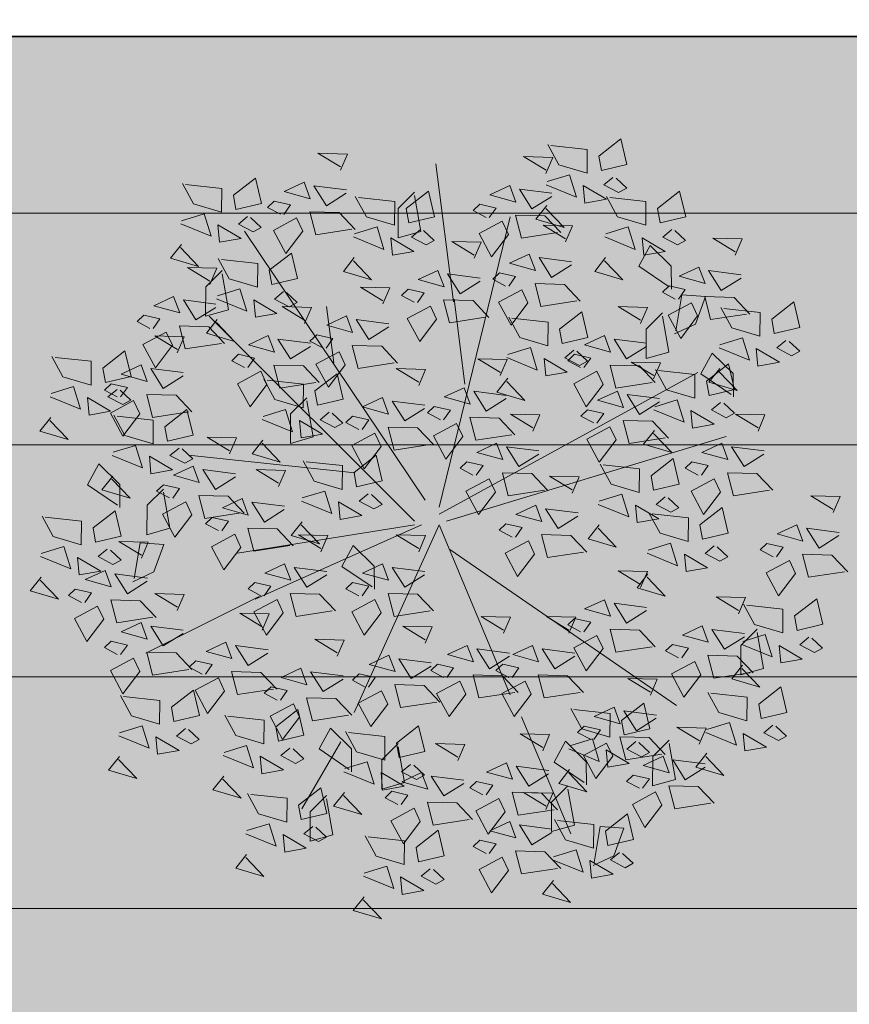
# Model space of a CAD drawing. Units: inches. Extents: x 1704 to 6393, y -157 to 1172.
# Tile 104 of 122: x 2627 to 2654, y 1002 to 1034. Entities that reach past the tile are written whole.
import ezdxf

# ---------------------------------------------------------------- set-up
doc = ezdxf.new("R2010")
doc.units = ezdxf.units.IN
doc.header["$MEASUREMENT"] = 0
for name, color, linetype, lineweight in [('A-ANNO-DIMS', 7, 'Continuous', 13), ('C-PROP', 7, 'Continuous', 35), ('L-DECK-PLNK-PATT', 250, 'Continuous', 13), ('L-shrub', 74, 'Continuous', 18)]:
    doc.layers.add(name, color=color, linetype=linetype, lineweight=lineweight)
doc.layers.add('L-DECK-PATT', color=35, linetype='Continuous', lineweight=13, true_color=0xa6725b)
doc.styles.get("Standard").update_dxf_attribs({"font": 'arial.ttf'})
doc.dimstyles.get("Standard").update_dxf_attribs({"dimtxt": 6, "dimasz": 2, "dimexe": 0.18, "dimexo": 0.0625, "dimgap": 0.09, "dimtad": 0, "dimtih": 1, "dimtoh": 1, "dimdec": 1, "dimzin": 0, "dimdsep": 46, "dimlunit": 3, "dimtxsty": 'Standard', "dimblk": 'ARCHTICK', "dimcen": 0.09, "dimadec": 0, "dimazin": 0, "dimtfac": 1, "dimtdec": 1, "dimtofl": 0, "dimtmove": 0, "dimatfit": 3, "dimfxl": 1, "dimtolj": 1, "dimtzin": 0, "dimarcsym": 0})

# ---------------------------------------------------------------- blocks, each defined once
blk = doc.blocks.new('flower shrub 2')
at = {"layer": 'L-shrub'}
for p, q in [((-106.23, 211.82), (-92.99, 218)), ((-93.69, 216.06), (-97.6, 193.26)), ((-112.6, 194.32), (-106.23, 211.82)), ((71.95, 198.59), (86.43, 202.67)), ((86.43, 202.67), (86.36, 184.05)), ((-97.6, 193.26), (-112.6, 194.32)), ((-81.12, 192.39), (-66.64, 196.47)), ((-66.64, 196.47), (-66.71, 177.85)), ((75.99, 175.82), (71.95, 198.59)), ((-77.07, 169.62), (-81.12, 192.39)), ((86.36, 184.05), (75.99, 173.75)), ((-66.71, 177.85), (-77.08, 167.55)), ((26.45, 165.53), (40.92, 169.61)), ((40.92, 169.61), (40.85, 150.99)), ((-145.24, 163.47), (-130.76, 167.54)), ((-141.2, 140.7), (-145.24, 163.47)), ((-130.76, 167.54), (-130.83, 148.93)), ((-88.72, 152.29), (-88.87, 166.9)), ((-87.4, 165.46), (-68.26, 152.47)), ((30.49, 142.76), (26.45, 165.53)), ((60.21, 144.02), (60.06, 158.64)), ((61.53, 157.19), (80.67, 144.21)), ((-75.44, 139.25), (-88.72, 152.29)), ((-68.26, 152.47), (-75.44, 139.25)), ((40.85, 150.99), (30.48, 140.69)), ((-130.83, 148.93), (-141.21, 138.63)), ((73.5, 130.99), (60.21, 144.02)), ((80.67, 144.21), (73.5, 130.99)), ((-201.09, 93.22), (-186.61, 97.3)), ((-186.61, 97.3), (-186.68, 78.69)), ((-197.05, 70.45), (-201.09, 93.22)), ((-186.68, 78.69), (-197.06, 68.38)), ((45.73, 28.33), (45.58, 42.95)), ((47.06, 41.5), (66.19, 28.51)), ((185.43, 32.08), (198.67, 38.26)), ((179.06, 14.59), (185.43, 32.08)), ((197.96, 36.32), (194.06, 13.53)), ((59.02, 15.29), (45.73, 28.33)), ((66.19, 28.51), (59.02, 15.29)), ((194.06, 13.53), (179.06, 14.59)), ((175.38, 4.39), (189.86, 8.47)), ((189.86, 8.47), (189.78, -10.15)), ((179.42, -18.38), (175.38, 4.39)), ((189.78, -10.15), (179.41, -20.45)), ((207.07, -23.32), (206.92, -8.7)), ((208.4, -10.15), (227.53, -23.13)), ((220.36, -36.35), (207.07, -23.32)), ((227.53, -23.13), (220.36, -36.35)), ((84.36, -53.46), (98.84, -49.38)), ((98.84, -49.38), (98.77, -68)), ((88.41, -76.23), (84.36, -53.46)), ((98.77, -68), (88.4, -78.3)), ((-181.81, -93.56), (-181.96, -78.94)), ((-180.48, -80.39), (-161.34, -93.38)), ((-168.52, -106.6), (-181.81, -93.56)), ((-161.34, -93.38), (-168.52, -106.6)), ((-141.1, -107.17), (-126.62, -103.09)), ((-126.62, -103.09), (-126.7, -121.71)), ((-137.06, -129.94), (-141.1, -107.17)), ((-157.94, -124.93), (-144.7, -118.75)), ((-145.41, -120.69), (-149.31, -143.48)), ((-126.7, -121.71), (-137.07, -132.01)), ((-164.31, -142.42), (-157.94, -124.93)), ((138.15, -134.03), (152.62, -129.95)), ((152.62, -129.95), (152.55, -148.57)), ((142.19, -156.8), (138.15, -134.03)), ((-149.31, -143.48), (-164.31, -142.42)), ((-142.51, -161.74), (-142.65, -147.12)), ((-141.18, -148.57), (-122.04, -161.55)), ((152.55, -148.57), (142.18, -158.87)), ((-129.22, -174.77), (-142.51, -161.74)), ((-122.04, -161.55), (-129.22, -174.77)), ((16.1, -183.61), (30.58, -179.53)), ((30.58, -179.53), (30.51, -198.15)), ((20.14, -206.38), (16.1, -183.61)), ((30.51, -198.15), (20.14, -208.45))]:
    blk.add_line(p, q, dxfattribs=at)
for points in [[(52.15, 237.83), (59.05, 246.56), (41.2, 251.84), (52.74, 239.81)], [(-67.82, 227.5), (-60.92, 236.23), (-78.77, 241.51), (-67.23, 229.48)], [(-39.32, 221.12), (-28.59, 235.29), (-20.71, 220.61), (-35.41, 212.74), (-39.32, 221.12)], [(29.03, 225.28), (27.99, 236.36), (14.33, 233.94), (29.03, 225.28)], [(52.02, 222.79), (37.77, 218.39), (33.35, 232.62), (52.6, 224.77)], [(-90.95, 214.95), (-91.98, 226.03), (-105.64, 223.61), (-90.95, 214.95)], [(10.23, 220.07), (15.95, 224.84), (6.62, 229.76), (1.48, 226.97), (8.24, 220.66)], [(126.62, 210.97), (133.52, 219.7), (115.67, 224.99), (127.2, 212.95)], [(-109.75, 209.74), (-104.02, 214.51), (-113.35, 219.43), (-118.49, 216.64), (-111.73, 210.33)], [(-67.96, 212.46), (-82.2, 208.06), (-86.62, 222.29), (-67.37, 214.44)], [(-70.39, 219.89), (-47.54, 223.41), (-43.79, 208.84), (-62.4, 209.34), (-72.46, 219.95)], [(19.2, 206.65), (5.18, 195.71), (1.34, 211.93), (17.57, 215.74), (19.2, 206.65)], [(49.53, 199.82), (26.54, 202.32), (26.68, 217.36), (44.53, 212.08), (51.52, 199.24)], [(-70.44, 189.49), (-93.43, 191.99), (-93.29, 207.03), (-75.44, 201.75), (-68.45, 188.91)], [(-27.19, 210.46), (-31.5, 204.37), (-21.21, 202.03), (-16.97, 206.05), (-25.13, 210.4)], [(103.49, 198.43), (102.46, 209.5), (88.8, 207.08), (103.49, 198.43)], [(-100.78, 196.32), (-114.8, 185.38), (-118.63, 201.6), (-102.4, 205.41), (-100.78, 196.32)], [(-66.87, 197.06), (-54.24, 204.99), (-46.3, 192.37), (-66.93, 195)], [(-44.01, 200.58), (-40.16, 190.14), (-27.58, 196), (-44.01, 200.58)], [(16.53, 190.13), (27.26, 204.31), (35.14, 189.63), (20.44, 181.76), (16.53, 190.13)], [(84.69, 193.22), (90.42, 197.99), (81.09, 202.9), (75.95, 200.11), (82.71, 193.8)], [(126.48, 195.93), (112.24, 191.53), (107.82, 205.76), (127.07, 197.91)], [(-136.54, 179.8), (-125.81, 193.98), (-117.93, 179.3), (-132.63, 171.43), (-136.54, 179.8)], [(-47.57, 123.92), (-79, 197.93)], [(-37.25, 183.93), (-26.52, 198.11), (-18.64, 183.43), (-33.34, 175.56), (-37.25, 183.93)], [(-14.54, 188.9), (8.31, 192.42), (12.06, 177.85), (-6.55, 178.35), (-16.61, 188.96)], [(93.66, 179.79), (79.64, 168.86), (75.81, 185.07), (92.04, 188.89), (93.66, 179.79)], [(124, 172.97), (101.01, 175.46), (101.15, 190.5), (119, 185.22), (125.98, 172.38)], [(-167.61, 178.57), (-144.76, 182.09), (-141.01, 167.52), (-159.62, 168.02), (-169.68, 178.63)], [(-68.32, 182.7), (-45.47, 186.22), (-41.72, 171.65), (-60.33, 172.15), (-70.39, 182.76)], [(-63.13, 182.49), (-67.54, 172.28), (-48.93, 171.78), (-63.18, 180.43)], [(64.56, 171.72), (71.46, 180.45), (53.61, 185.73), (65.15, 173.7)], [(66.94, 139.62), (91.63, 182.23)], [(28.66, 179.47), (24.35, 173.38), (34.64, 171.04), (38.88, 175.06), (30.72, 179.41)], [(141.1, 161.39), (148, 170.12), (130.14, 175.4), (141.68, 163.37)], [(-124.41, 169.14), (-128.72, 163.05), (-118.43, 160.71), (-114.19, 164.73), (-122.34, 169.08)], [(-78.16, 157.26), (-71.26, 165.99), (-89.12, 171.27), (-77.58, 159.24)], [(-25.12, 173.27), (-29.43, 167.19), (-19.14, 164.84), (-14.9, 168.86), (-23.06, 173.21)], [(-11.02, 166.07), (1.61, 174), (9.54, 161.38), (-11.08, 164.01)], [(11.84, 169.59), (15.69, 159.15), (28.27, 165.01), (11.84, 169.59)], [(41.44, 159.17), (40.4, 170.25), (26.74, 167.83), (41.44, 159.17)], [(-164.09, 155.74), (-151.46, 163.67), (-143.52, 151.05), (-164.15, 153.68)], [(-105.51, 148.81), (-94.78, 162.99), (-86.9, 148.31), (-101.6, 140.44), (-105.51, 148.81)], [(-64.8, 159.87), (-52.17, 167.8), (-44.24, 155.19), (-64.86, 157.81)], [(-41.95, 163.39), (-38.09, 152.95), (-25.52, 158.81), (-41.95, 163.39)], [(22.64, 153.96), (28.36, 158.73), (19.03, 163.65), (13.89, 160.86), (20.65, 154.55)], [(64.43, 156.68), (50.18, 152.28), (45.76, 166.51), (65.01, 158.66)], [(207.29, 148.99), (214.19, 157.72), (196.34, 163.01), (207.88, 150.97)], [(-165.04, 146.93), (-158.14, 155.66), (-175.99, 160.94), (-164.45, 148.91)], [(-141.23, 159.26), (-137.38, 148.82), (-124.8, 154.68), (-141.23, 159.26)], [(117.97, 148.84), (116.93, 159.92), (103.28, 157.5), (117.97, 148.84)], [(140.96, 146.35), (126.72, 141.95), (122.3, 156.18), (141.55, 148.33)], [(-136.58, 147.58), (-113.73, 151.1), (-109.98, 136.53), (-128.59, 137.03), (-138.65, 147.64)], [(-101.29, 144.71), (-102.33, 155.79), (-115.98, 153.37), (-101.29, 144.71)], [(-78.3, 142.22), (-92.54, 137.81), (-96.96, 152.05), (-77.71, 144.2)], [(-7.28, 151.5), (-11.69, 141.29), (6.92, 140.79), (-7.33, 149.44)], [(61.95, 133.71), (38.95, 136.21), (39.09, 151.25), (56.94, 145.97), (63.93, 133.13)], [(99.17, 143.63), (104.9, 148.4), (95.57, 153.32), (90.43, 150.53), (97.19, 144.22)], [(-188.17, 134.38), (-189.2, 145.46), (-202.86, 143.04), (-188.17, 134.38)], [(-120.09, 139.5), (-114.36, 144.27), (-123.69, 149.19), (-128.83, 146.4), (-122.07, 140.09)], [(-61.06, 145.31), (-65.47, 135.09), (-46.86, 134.59), (-61.11, 143.24)], [(31.61, 140.54), (17.59, 129.6), (13.76, 145.82), (29.99, 149.63), (31.61, 140.54)], [(184.16, 136.45), (183.13, 147.53), (169.47, 145.1), (184.16, 136.45)], [(207.15, 133.95), (192.91, 129.55), (188.49, 143.78), (207.74, 135.93)], [(-206.97, 129.17), (-201.24, 133.94), (-210.57, 138.86), (-215.71, 136.07), (-208.95, 129.76)], [(-165.18, 131.89), (-179.42, 127.48), (-183.84, 141.72), (-164.59, 133.87)], [(-160.34, 141.17), (-164.76, 130.96), (-146.15, 130.46), (-160.4, 139.11)], [(-93.39, 138.15), (-97.69, 132.06), (-87.4, 129.72), (-83.16, 133.74), (-91.32, 138.09)], [(108.14, 130.21), (94.12, 119.27), (90.29, 135.49), (106.52, 139.3), (108.14, 130.21)], [(93.06, 124.02), (103.79, 138.2), (111.67, 123.52), (96.98, 115.65), (93.06, 124.02)], [(138.48, 123.38), (115.49, 125.88), (115.63, 140.92), (133.48, 135.64), (140.46, 122.8)], [(165.36, 131.24), (171.09, 136.01), (161.76, 140.92), (156.62, 138.13), (163.38, 131.82)], [(-133.06, 124.75), (-120.43, 132.68), (-112.5, 120.06), (-133.12, 122.69)], [(-111.12, 126.07), (-125.14, 115.14), (-128.97, 131.36), (-112.74, 135.17), (-111.12, 126.07)], [(-80.78, 119.25), (-103.77, 121.75), (-103.63, 136.79), (-85.78, 131.5), (-78.8, 118.66)], [(-198, 115.75), (-212.02, 104.81), (-215.85, 121.03), (-199.62, 124.84), (-198, 115.75)], [(-167.66, 108.92), (-190.65, 111.42), (-190.51, 126.46), (-172.66, 121.17), (-165.67, 108.33)], [(-110.21, 128.27), (-106.35, 117.83), (-93.78, 123.69), (-110.21, 128.27)], [(37.21, 115.75), (47.94, 129.93), (55.82, 115.25), (41.13, 107.38), (37.21, 115.75)], [(61.99, 122.79), (84.85, 126.31), (88.59, 111.74), (69.98, 112.24), (59.92, 122.85)], [(174.33, 117.81), (160.31, 106.88), (156.48, 123.09), (172.71, 126.91), (174.33, 117.81)], [(204.67, 110.99), (181.68, 113.48), (181.82, 128.52), (199.67, 123.24), (206.65, 110.4)], [(-53.8, 109.56), (-43.07, 123.73), (-35.19, 109.05), (-49.89, 101.18), (-53.8, 109.56)], [(-12.43, 109.56), (-1.7, 123.73), (6.18, 109.05), (-8.52, 101.18), (-12.43, 109.56)], [(4.49, 2.24), (58.38, 121.09)], [(140.64, 107.49), (151.37, 121.67), (159.25, 106.99), (144.55, 99.12), (140.64, 107.49)], [(-2.25, 17.94), (-145.94, 116.61)], [(6.14, 114.53), (29, 118.04), (32.74, 103.47), (14.13, 103.98), (4.07, 114.58)], [(105.19, 113.36), (100.89, 107.27), (111.17, 104.93), (115.42, 108.95), (107.26, 113.3)], [(-161.36, 97.16), (-150.63, 111.34), (-142.75, 96.66), (-157.45, 88.79), (-161.36, 97.16)], [(-129.32, 110.18), (-133.73, 99.97), (-115.12, 99.47), (-129.37, 108.12)], [(-84.87, 108.33), (-62.02, 111.85), (-58.27, 97.28), (-76.88, 97.78), (-86.94, 108.38)], [(-43.5, 108.33), (-20.65, 111.85), (-16.9, 97.28), (-35.51, 97.78), (-45.57, 108.38)], [(4.49, 2.24), (-40.41, 109.88)], [(65.51, 99.96), (78.14, 107.89), (86.08, 95.27), (65.46, 97.9)], [(109.57, 106.26), (132.42, 109.78), (136.17, 95.21), (117.56, 95.71), (107.5, 106.32)], [(194.42, 95.09), (205.15, 109.27), (213.03, 94.59), (198.33, 86.72), (194.42, 95.09)], [(-187.79, 91.15), (-180.89, 99.88), (-198.75, 105.16), (-187.21, 93.13)], [(49.34, 105.09), (45.04, 99.01), (55.32, 96.67), (59.57, 100.68), (51.41, 105.04)], [(88.37, 103.48), (92.23, 93.04), (104.8, 98.9), (88.37, 103.48)], [(-192.43, 95.93), (-169.58, 99.45), (-165.83, 84.88), (-184.44, 85.38), (-194.5, 95.99)], [(-99.31, 80.63), (-88.58, 94.81), (-80.7, 80.13), (-95.39, 72.26), (-99.31, 80.63)], [(-41.67, 98.9), (-45.98, 92.81), (-35.69, 90.47), (-31.45, 94.49), (-39.6, 98.84)], [(-0.3, 98.9), (-4.61, 92.81), (5.68, 90.47), (9.92, 94.49), (1.76, 98.84)], [(9.66, 91.7), (22.29, 99.62), (30.23, 87.01), (9.61, 89.63)], [(32.52, 95.21), (36.38, 84.78), (48.95, 90.64), (32.52, 95.21)], [(152.77, 96.83), (148.46, 90.75), (158.75, 88.4), (162.99, 92.42), (154.83, 96.77)], [(163.35, 93.87), (186.2, 97.38), (189.95, 82.82), (171.34, 83.32), (161.28, 93.92)], [(-210.92, 78.6), (-211.96, 89.68), (-225.62, 87.26), (-210.92, 78.6)], [(-81.35, 85.5), (-68.72, 93.43), (-60.78, 80.81), (-81.41, 83.43)], [(-58.49, 89.02), (-54.64, 78.58), (-42.06, 84.44), (-58.49, 89.02)], [(-39.98, 85.5), (-27.35, 93.43), (-19.41, 80.81), (-40.04, 83.43)], [(-17.12, 89.02), (-13.27, 78.58), (-0.69, 84.44), (-17.12, 89.02)], [(113.09, 83.43), (125.72, 91.36), (133.65, 78.75), (113.03, 81.37)], [(-229.72, 73.39), (-223.99, 78.16), (-233.32, 83.08), (-238.46, 80.29), (-231.7, 73.98)], [(-187.93, 76.11), (-202.17, 71.7), (-206.59, 85.94), (-187.34, 78.09)], [(-149.23, 86.5), (-153.54, 80.42), (-143.25, 78.07), (-139.01, 82.09), (-147.17, 86.44)], [(-130.38, 79.41), (-107.52, 82.92), (-103.78, 68.35), (-122.39, 68.86), (-132.45, 79.46)], [(69.26, 85.39), (64.84, 75.18), (83.45, 74.68), (69.2, 83.33)], [(118.58, 47.68), (190.43, 83.56)], [(135.94, 86.95), (139.8, 76.51), (152.38, 82.37), (135.94, 86.95)], [(206.55, 84.43), (202.24, 78.35), (212.53, 76.01), (216.77, 80.02), (208.61, 84.38)], [(-188.91, 73.1), (-176.28, 81.03), (-168.35, 68.42), (-188.97, 71.04)], [(-166.05, 76.62), (-162.2, 66.18), (-149.62, 72.04), (-166.05, 76.62)], [(13.41, 77.13), (8.99, 66.92), (27.6, 66.41), (13.35, 75.06)], [(166.87, 71.04), (179.5, 78.96), (187.44, 66.35), (166.81, 68.97)], [(217.17, 62.04), (227.9, 76.22), (235.78, 61.54), (221.08, 53.67), (217.17, 62.04)], [(-220.75, 59.96), (-234.77, 49.03), (-238.6, 65.25), (-222.37, 69.06), (-220.75, 59.96)], [(-190.41, 53.14), (-213.4, 55.64), (-213.26, 70.68), (-195.41, 65.39), (-188.43, 52.55)], [(-87.18, 69.97), (-91.48, 63.89), (-81.2, 61.54), (-76.95, 65.56), (-85.11, 69.92)], [(-77.6, 70.93), (-82.02, 60.72), (-63.41, 60.22), (-77.66, 68.87)], [(-36.23, 70.93), (-40.65, 60.72), (-22.04, 60.22), (-36.29, 68.87)], [(41.35, 57.91), (52.08, 72.09), (59.96, 57.41), (45.26, 49.54), (41.35, 57.91)], [(103.41, 57.91), (114.13, 72.09), (122.01, 57.41), (107.32, 49.54), (103.41, 57.91)], [(116.83, 68.87), (112.42, 58.65), (131.03, 58.15), (116.78, 66.8)], [(189.73, 74.55), (193.58, 64.12), (206.16, 69.98), (189.73, 74.55)], [(-126.86, 56.58), (-114.23, 64.5), (-106.29, 51.89), (-126.91, 54.51)], [(186.1, 60.81), (208.96, 64.33), (212.7, 49.76), (194.09, 50.26), (184.03, 60.87)], [(-185.17, 58.54), (-189.58, 48.32), (-170.97, 47.82), (-185.22, 56.47)], [(-104, 60.09), (-100.14, 49.66), (-87.57, 55.52), (-104, 60.09)], [(10.28, 56.68), (33.14, 60.2), (36.88, 45.63), (18.27, 46.13), (8.21, 56.74)], [(72.33, 56.68), (95.19, 60.2), (98.94, 45.63), (80.33, 46.13), (70.27, 56.74)], [(170.61, 56.47), (166.2, 46.26), (184.81, 45.75), (170.56, 54.41)], [(229.3, 51.38), (225, 45.3), (235.28, 42.95), (239.53, 46.97), (231.37, 51.32)], [(-221.35, 33.12), (-210.62, 47.29), (-202.74, 32.61), (-217.44, 24.74), (-221.35, 33.12)], [(-127.81, 33.3), (-120.91, 42.03), (-138.76, 47.31), (-127.22, 35.28)], [(15.72, 2.24), (121.24, 49.33)], [(53.48, 47.25), (49.18, 41.16), (59.46, 38.82), (63.71, 42.84), (55.55, 47.19)], [(115.53, 47.25), (111.23, 41.16), (121.51, 38.82), (125.76, 42.84), (117.6, 47.19)], [(189.62, 37.98), (202.25, 45.91), (210.19, 33.29), (189.57, 35.92)], [(256.93, 35.37), (263.83, 44.1), (245.98, 49.38), (257.52, 37.35)], [(-123.11, 42.01), (-127.53, 31.79), (-108.92, 31.29), (-123.17, 39.94)], [(13.8, 33.85), (26.43, 41.78), (34.37, 29.16), (13.74, 31.79)], [(75.86, 33.85), (88.48, 41.78), (96.42, 29.16), (75.8, 31.79)], [(212.48, 41.5), (216.34, 31.06), (228.91, 36.92), (212.48, 41.5)], [(-252.42, 31.89), (-229.56, 35.41), (-225.82, 20.84), (-244.43, 21.34), (-254.49, 31.94)], [(-150.93, 20.75), (-151.97, 31.83), (-165.63, 29.41), (-150.93, 20.75)], [(-55.87, 20.72), (-45.14, 34.9), (-37.26, 20.22), (-51.96, 12.35), (-55.87, 20.72)], [(36.66, 37.37), (40.51, 26.93), (53.09, 32.79), (36.66, 37.37)], [(98.71, 37.37), (102.57, 26.93), (115.14, 32.79), (98.71, 37.37)], [(233.81, 22.82), (232.77, 33.9), (219.11, 31.48), (233.81, 22.82)], [(-169.73, 15.55), (-164.01, 20.31), (-173.34, 25.23), (-178.48, 22.44), (-171.72, 16.13)], [(-127.94, 18.26), (-142.19, 13.86), (-146.61, 28.09), (-127.36, 20.24)], [(130.3, 16.59), (141.02, 30.77), (148.91, 16.09), (134.21, 8.22), (130.3, 16.59)], [(215.01, 17.61), (220.73, 22.38), (211.4, 27.3), (206.26, 24.51), (213.02, 18.2)], [(256.8, 20.33), (242.55, 15.92), (238.13, 30.16), (257.38, 22.31)], [(-209.22, 22.46), (-213.52, 16.37), (-203.24, 14.03), (-198.99, 18.05), (-207.15, 22.4)], [(-86.94, 19.49), (-64.08, 23.01), (-60.34, 8.44), (-78.95, 8.94), (-89.01, 19.55)], [(17.55, 19.28), (13.13, 9.07), (31.74, 8.57), (17.49, 17.22)], [(20.21, 2.24), (132.47, 20.18)], [(79.6, 19.28), (75.19, 9.07), (93.8, 8.57), (79.54, 17.22)], [(99.22, 15.36), (122.08, 18.88), (125.83, 4.31), (107.22, 4.81), (97.16, 15.42)], [(193.37, 23.42), (188.95, 13.2), (207.56, 12.7), (193.31, 21.35)], [(-248.9, 9.06), (-236.27, 16.99), (-228.33, 4.37), (-248.95, 7)], [(-226.04, 12.58), (-222.18, 2.14), (-209.61, 8), (-226.04, 12.58)], [(-130.42, -4.7), (-153.42, -2.21), (-153.28, 12.83), (-135.43, 7.55), (-128.44, -5.29)], [(-96.78, 2.31), (-89.88, 11.04), (-107.73, 16.33), (-96.19, 4.29)], [(91.45, 0.25), (98.35, 8.98), (80.5, 14.26), (92.04, 2.23)], [(223.98, 4.18), (209.96, -6.75), (206.13, 9.47), (222.35, 13.28), (223.98, 4.18)], [(254.32, -2.64), (231.32, -0.14), (231.46, 14.9), (249.31, 9.61), (256.3, -3.23)], [(-160.76, 2.12), (-174.78, -8.81), (-178.61, 7.4), (-162.38, 11.22), (-160.76, 2.12)], [(-43.74, 10.06), (-48.04, 3.98), (-37.76, 1.63), (-33.51, 5.65), (-41.67, 10)], [(161.32, -4.07), (172.05, 10.11), (179.93, -4.57), (165.24, -12.44), (161.32, -4.07)], [(0, 0), (-177.37, -53.82)], [(-119.91, -10.23), (-120.94, 0.84), (-134.6, -1.58), (-119.91, -10.23)], [(-83.42, -3.34), (-70.79, 4.59), (-62.85, -8.02), (-83.47, -5.4)], [(-60.56, 0.18), (-56.71, -10.26), (-44.13, -4.4), (-60.56, 0.18)], [(20.21, 0), (150.43, -130.06)], [(102.75, -7.47), (115.38, 0.46), (123.31, -12.16), (102.69, -9.53)], [(142.42, 5.93), (138.12, -0.16), (148.4, -2.5), (152.65, 1.52), (144.49, 5.87)], [(-245.15, -5.51), (-249.57, -15.72), (-230.96, -16.22), (-245.21, -7.57)], [(-173.77, -18.53), (-163.04, -4.35), (-155.16, -19.03), (-169.86, -26.9), (-173.77, -18.53)], [(4.49, -4.48), (-159.41, -94.18)], [(-138.71, -15.44), (-132.98, -10.67), (-142.31, -5.76), (-147.45, -8.55), (-140.69, -14.86)], [(-96.92, -12.73), (-111.16, -17.13), (-115.58, -2.9), (-96.33, -10.75)], [(-31.05, -18.53), (-20.32, -4.35), (-12.44, -19.03), (-27.13, -26.9), (-31.05, -18.53)], [(68.33, -12.3), (67.29, -1.22), (53.63, -3.64), (68.33, -12.3)], [(91.32, -14.79), (77.07, -19.2), (72.66, -4.96), (91.9, -12.81)], [(125.6, -3.95), (129.46, -14.39), (142.03, -8.53), (125.6, -3.95)], [(130.25, -5.3), (153.11, -1.78), (156.85, -16.35), (138.24, -15.85), (128.18, -5.24)], [(4.49, -8.97), (-40.41, -192.85)], [(49.53, -17.51), (55.25, -12.74), (45.92, -7.82), (40.78, -10.61), (47.54, -16.92)], [(-204.84, -19.76), (-181.99, -16.24), (-178.24, -30.81), (-196.85, -30.31), (-206.91, -19.7)], [(-99.4, -35.69), (-122.39, -33.2), (-122.25, -18.16), (-104.4, -23.44), (-97.41, -36.28)], [(-79.67, -17.9), (-84.09, -28.12), (-65.48, -28.62), (-79.73, -19.97)], [(-62.12, -19.76), (-39.26, -16.24), (-35.52, -30.81), (-54.13, -30.31), (-64.19, -19.7)], [(13.47, -13.45), (127.98, -183.88)], [(173.45, -14.73), (169.15, -20.81), (179.43, -23.16), (183.68, -19.14), (175.52, -14.79)], [(211.43, -28.68), (218.32, -19.95), (200.47, -14.66), (212.01, -26.7)], [(-129.74, -28.87), (-143.76, -39.8), (-147.59, -23.59), (-131.36, -19.77), (-129.74, -28.87)], [(58.5, -30.94), (44.48, -41.87), (40.65, -25.65), (56.88, -21.84), (58.5, -30.94)], [(88.84, -37.76), (65.84, -35.27), (65.98, -20.22), (83.83, -25.51), (90.82, -38.35)], [(106.49, -22.04), (102.08, -32.25), (120.69, -32.75), (106.44, -24.1)], [(133.77, -28.13), (146.4, -20.2), (154.34, -32.82), (133.72, -30.19)], [(156.63, -24.61), (160.49, -35.05), (173.06, -29.19), (156.63, -24.61)], [(-161.65, -29.19), (-165.95, -35.28), (-155.67, -37.62), (-151.42, -33.6), (-159.58, -29.25)], [(-18.92, -29.19), (-23.22, -35.28), (-12.94, -37.62), (-8.69, -33.6), (-16.85, -29.25)], [(57.96, -30.81), (163.48, -42.02)], [(188.3, -41.22), (187.26, -30.14), (173.6, -32.57), (188.3, -41.22)], [(-201.32, -42.59), (-188.69, -34.66), (-180.76, -47.28), (-201.38, -44.65)], [(-107.58, -51.59), (-96.85, -37.41), (-88.97, -52.09), (-103.67, -59.96), (-107.58, -51.59)], [(-58.6, -42.59), (-45.97, -34.66), (-38.03, -47.28), (-58.65, -44.65)], [(41.35, -47.45), (52.08, -33.28), (59.96, -47.96), (45.26, -55.83), (41.35, -47.45)], [(116.28, -51.4), (123.17, -42.67), (105.32, -37.39), (116.86, -49.42)], [(169.5, -46.43), (175.23, -41.66), (165.89, -36.75), (160.76, -39.54), (167.52, -45.85)], [(211.29, -43.72), (197.04, -48.12), (192.63, -33.89), (211.88, -41.74)], [(-178.47, -39.07), (-174.61, -49.51), (-162.04, -43.65), (-178.47, -39.07)], [(-131.94, -57.6), (-125.04, -48.87), (-142.9, -43.59), (-131.36, -55.62)], [(-35.74, -39.07), (-31.88, -49.51), (-19.31, -43.65), (-35.74, -39.07)], [(-10.36, -53.65), (0.37, -39.48), (8.25, -54.15), (-6.45, -62.02), (-10.36, -53.65)], [(137.52, -42.69), (133.1, -52.91), (151.71, -53.41), (137.46, -44.76)], [(-138.65, -52.81), (-115.8, -49.3), (-112.05, -63.87), (-130.66, -63.36), (-140.72, -52.76)], [(10.28, -48.68), (33.14, -45.17), (36.88, -59.73), (18.27, -59.23), (8.21, -48.63)], [(208.81, -66.68), (185.82, -64.19), (185.95, -49.15), (203.81, -54.43), (210.79, -67.27)], [(-41.43, -54.88), (-18.58, -51.36), (-14.83, -65.93), (-33.44, -65.43), (-43.5, -54.82)], [(93.15, -63.95), (92.11, -52.87), (78.45, -55.29), (93.15, -63.95)], [(178.47, -59.86), (164.45, -70.79), (160.62, -54.58), (176.85, -50.76), (178.47, -59.86)], [(194.42, -68.11), (205.15, -53.94), (213.03, -68.62), (198.33, -76.49), (194.42, -68.11)], [(250.73, -65.86), (257.63, -57.13), (239.78, -51.85), (251.31, -63.88)], [(-197.58, -57.16), (-201.99, -67.37), (-183.38, -67.87), (-197.63, -59.22)], [(-155.07, -70.15), (-156.11, -59.07), (-169.77, -61.49), (-155.07, -70.15)], [(-95.45, -62.25), (-99.76, -68.33), (-89.47, -70.68), (-85.23, -66.66), (-93.39, -62.3)], [(-54.85, -57.16), (-59.27, -67.37), (-40.66, -67.87), (-54.91, -59.22)], [(53.48, -58.12), (49.18, -64.2), (59.46, -66.54), (63.71, -62.52), (55.55, -58.17)], [(74.35, -69.16), (80.08, -64.39), (70.74, -59.47), (65.6, -62.26), (72.37, -68.57)], [(116.14, -66.44), (101.89, -70.85), (97.48, -56.61), (116.73, -64.46)], [(-173.87, -75.36), (-168.14, -70.59), (-177.47, -65.67), (-182.61, -68.46), (-175.85, -74.77)], [(-132.08, -72.64), (-146.33, -77.04), (-150.74, -62.81), (-131.49, -70.66)], [(-135.13, -75.64), (-122.5, -67.72), (-114.56, -80.33), (-135.19, -77.71)], [(1.77, -64.31), (-2.54, -70.4), (7.75, -72.74), (11.99, -68.72), (3.83, -64.37)], [(13.8, -71.51), (26.43, -63.59), (34.37, -76.2), (13.74, -73.58)], [(36.66, -67.99), (40.51, -78.43), (53.09, -72.57), (36.66, -67.99)], [(163.35, -69.34), (186.2, -65.83), (189.95, -80.39), (171.34, -79.89), (161.28, -69.29)], [(227.6, -78.41), (226.56, -67.33), (212.91, -69.75), (227.6, -78.41)], [(-112.27, -72.13), (-108.42, -82.56), (-95.84, -76.7), (-112.27, -72.13)], [(-99.31, -86.71), (-88.58, -72.53), (-80.7, -87.21), (-95.39, -95.08), (-99.31, -86.71)], [(-37.91, -77.71), (-25.28, -69.78), (-17.35, -82.4), (-37.97, -79.77)], [(-15.06, -74.19), (-11.2, -84.63), (1.38, -78.77), (-15.06, -74.19)], [(83.32, -82.58), (69.3, -93.52), (65.47, -77.3), (81.7, -73.49), (83.32, -82.58)], [(113.66, -89.41), (90.67, -86.91), (90.8, -71.87), (108.65, -77.16), (115.64, -90)], [(113.75, -86.71), (124.48, -72.53), (132.36, -87.21), (117.66, -95.08), (113.75, -86.71)], [(208.8, -83.62), (214.53, -78.85), (205.2, -73.93), (200.06, -76.72), (206.82, -83.03)], [(250.59, -80.9), (236.35, -85.31), (231.93, -71.07), (251.18, -78.92)], [(-164.9, -88.78), (-178.92, -99.72), (-182.75, -83.5), (-166.52, -79.68), (-164.9, -88.78)], [(-134.56, -95.61), (-157.55, -93.11), (-157.42, -78.07), (-139.56, -83.35), (-132.58, -96.19)], [(-38.86, -90.66), (-31.96, -81.92), (-49.81, -76.64), (-38.27, -88.67)], [(206.55, -78.77), (202.24, -84.86), (212.53, -87.2), (216.77, -83.18), (208.61, -78.83)], [(-173.31, -96.85), (-166.41, -88.12), (-184.27, -82.84), (-172.73, -94.87)], [(-130.38, -87.94), (-107.52, -84.42), (-103.78, -98.99), (-122.39, -98.48), (-132.45, -87.88)], [(-4.91, -140.69), (-11.65, -86.87)], [(17.55, -86.08), (13.13, -96.29), (31.74, -96.8), (17.49, -88.14)], [(64.1, -99.1), (74.83, -84.93), (82.71, -99.61), (68.02, -107.48), (64.1, -99.1)], [(82.68, -87.94), (105.53, -84.42), (109.28, -98.99), (90.67, -98.48), (80.61, -87.88)], [(166.87, -92.17), (179.5, -84.24), (187.44, -96.86), (166.81, -94.24)], [(248.11, -103.87), (225.12, -101.38), (225.26, -86.33), (243.11, -91.62), (250.09, -104.46)], [(-131.39, -90.21), (-135.8, -100.43), (-117.19, -100.93), (-131.44, -92.28)], [(-61.99, -103.2), (-63.02, -92.12), (-76.68, -94.54), (-61.99, -103.2)], [(-34.17, -92.28), (-38.58, -102.49), (-19.97, -102.99), (-34.22, -94.34)], [(189.73, -88.65), (193.58, -99.09), (206.16, -93.23), (189.73, -88.65)], [(217.77, -97.05), (203.75, -107.98), (199.92, -91.76), (216.15, -87.95), (217.77, -97.05)], [(-196.44, -109.4), (-197.48, -98.32), (-211.14, -100.74), (-196.44, -109.4)], [(-87.18, -97.37), (-91.48, -103.45), (-81.2, -105.8), (-76.95, -101.78), (-85.11, -97.42)], [(-80.79, -108.41), (-75.06, -103.64), (-84.39, -98.73), (-89.53, -101.51), (-82.77, -107.82)], [(-39, -105.7), (-53.24, -110.1), (-57.66, -95.86), (-38.41, -103.72)], [(33.03, -100.33), (55.89, -96.81), (59.63, -111.38), (41.02, -110.88), (30.96, -100.28)], [(125.88, -97.37), (121.57, -103.45), (131.86, -105.8), (136.1, -101.78), (127.94, -97.42)], [(173.73, -111.5), (184.46, -97.32), (192.34, -112), (177.65, -119.87), (173.73, -111.5)], [(-215.24, -114.61), (-209.51, -109.84), (-218.84, -104.92), (-223.98, -107.71), (-217.22, -114.02)], [(-173.45, -111.89), (-187.7, -116.3), (-192.11, -102.06), (-172.86, -109.91)], [(-126.86, -110.76), (-114.23, -102.84), (-106.29, -115.45), (-126.91, -112.83)], [(71.43, -100.32), (75.92, -136.2)], [(86.2, -110.76), (98.83, -102.84), (106.76, -115.45), (86.14, -112.83)], [(-104, -107.25), (-100.14, -117.69), (-87.57, -111.82), (-104, -107.25)], [(-41.48, -128.66), (-64.47, -126.17), (-64.33, -111.13), (-46.48, -116.41), (-39.5, -129.25)], [(76.23, -109.76), (71.93, -115.85), (82.21, -118.19), (86.46, -114.17), (78.3, -109.82)], [(109.05, -107.25), (112.91, -117.69), (125.48, -111.82), (109.05, -107.25)], [(142.66, -112.73), (165.52, -109.21), (169.26, -123.78), (150.65, -123.28), (140.59, -112.67)], [(170.61, -106.74), (166.2, -116.95), (184.81, -117.46), (170.56, -108.8)], [(-175.93, -134.86), (-198.92, -132.36), (-198.79, -117.32), (-180.93, -122.61), (-173.95, -135.45)], [(-159.29, -130.09), (-148.56, -115.91), (-140.68, -130.59), (-155.38, -138.46), (-159.29, -130.09)], [(-71.82, -121.84), (-85.84, -132.77), (-89.67, -116.56), (-73.44, -112.74), (-71.82, -121.84)], [(6.19, -128.03), (16.91, -113.85), (24.8, -128.53), (10.1, -136.4), (6.19, -128.03)], [(36.55, -123.16), (49.18, -115.23), (57.12, -127.85), (36.5, -125.22)], [(145.23, -127.84), (152.13, -119.11), (134.28, -113.83), (145.82, -125.86)], [(-206.27, -128.04), (-220.29, -138.97), (-224.12, -122.75), (-207.89, -118.94), (-206.27, -128.04)], [(-51.73, -138.36), (-41, -124.18), (-33.12, -138.86), (-47.82, -146.73), (-51.73, -138.36)], [(59.41, -119.64), (63.27, -130.08), (75.84, -124.22), (59.41, -119.64)], [(185.86, -122.16), (181.56, -128.24), (191.84, -130.59), (196.09, -126.57), (187.93, -122.22)], [(-190.37, -131.32), (-167.51, -127.8), (-163.76, -142.37), (-182.37, -141.87), (-192.43, -131.26)], [(-123.11, -125.33), (-127.53, -135.55), (-108.92, -136.05), (-123.17, -127.4)], [(-24.89, -129.25), (-2.03, -125.74), (1.72, -140.31), (-16.89, -139.8), (-26.95, -129.2)], [(89.94, -125.33), (85.53, -135.55), (104.14, -136.05), (89.89, -127.4)], [(122.11, -140.39), (121.07, -129.31), (107.41, -131.73), (122.11, -140.39)], [(146.18, -135.56), (158.81, -127.63), (166.75, -140.24), (146.13, -137.62)], [(-82.8, -139.58), (-59.95, -136.07), (-56.2, -150.64), (-74.81, -150.13), (-84.87, -139.53)], [(103.31, -145.6), (109.03, -140.83), (99.7, -135.91), (94.56, -138.7), (101.33, -145.01)], [(145.1, -142.88), (130.85, -147.29), (126.44, -133.05), (145.68, -140.9)], [(169.04, -132.04), (172.9, -142.48), (185.47, -136.62), (169.04, -132.04)], [(-147.17, -140.75), (-151.47, -146.84), (-141.19, -149.18), (-136.94, -145.16), (-145.1, -140.81)], [(-4.49, -139.03), (6.74, -226.49)], [(18.31, -138.69), (14.01, -144.77), (24.29, -147.12), (28.54, -143.1), (20.38, -138.74)], [(40.3, -137.73), (35.89, -147.94), (54.49, -148.44), (40.24, -139.79)], [(-186.84, -154.15), (-174.21, -146.22), (-166.28, -158.84), (-186.9, -156.21)], [(-39.6, -149.02), (-43.91, -155.1), (-33.62, -157.44), (-29.38, -153.43), (-37.54, -149.07)], [(-21.36, -152.08), (-8.73, -144.16), (-0.8, -156.77), (-21.42, -154.15)], [(1.49, -148.57), (5.35, -159), (17.92, -153.14), (1.49, -148.57)], [(142.62, -165.85), (119.63, -163.35), (119.76, -148.31), (137.61, -153.6), (144.6, -166.44)], [(-163.99, -150.63), (-160.13, -161.07), (-147.56, -155.21), (-163.99, -150.63)], [(-100.92, -167.09), (-94.02, -158.36), (-111.87, -153.08), (-100.33, -165.11)], [(-79.28, -162.41), (-66.65, -154.49), (-58.72, -167.1), (-79.34, -164.48)], [(58.36, -167.09), (65.26, -158.36), (47.41, -153.08), (58.94, -165.11)], [(112.28, -159.02), (98.26, -169.96), (94.43, -153.74), (110.66, -149.93), (112.28, -159.02)], [(149.93, -150.12), (145.52, -160.34), (164.12, -160.84), (149.87, -152.19)], [(-56.42, -158.9), (-52.57, -169.33), (-39.99, -163.47), (-56.42, -158.9)], [(167.99, -175.36), (174.89, -166.63), (157.04, -161.34), (168.57, -173.38)], [(-39.32, -181.74), (-28.59, -167.56), (-20.71, -182.24), (-35.41, -190.11), (-39.32, -181.74)], [(-17.62, -166.65), (-22.03, -176.87), (-3.42, -177.37), (-17.67, -168.72)], [(-183.1, -168.72), (-187.51, -178.93), (-168.9, -179.43), (-183.15, -170.78)], [(-124.04, -179.64), (-125.08, -168.56), (-138.74, -170.98), (-124.04, -179.64)], [(-101.05, -182.14), (-115.3, -186.54), (-119.71, -172.3), (-100.47, -180.15)], [(35.23, -179.64), (34.2, -168.56), (20.54, -170.98), (35.23, -179.64)], [(58.22, -182.14), (43.98, -186.54), (39.56, -172.3), (58.81, -180.15)], [(90.99, -183.81), (101.72, -169.63), (109.6, -184.31), (94.91, -192.18), (90.99, -183.81)], [(-142.84, -184.85), (-137.12, -180.08), (-146.45, -175.17), (-151.59, -177.95), (-144.83, -184.26)], [(-75.54, -176.98), (-79.95, -187.19), (-61.34, -187.7), (-75.59, -179.05)], [(-70.39, -182.97), (-47.54, -179.45), (-43.79, -194.02), (-62.4, -193.52), (-72.46, -182.91)], [(16.43, -184.85), (22.16, -180.08), (12.83, -175.17), (7.69, -177.95), (14.45, -184.26)], [(144.86, -187.9), (143.83, -176.83), (130.17, -179.25), (144.86, -187.9)], [(167.85, -190.4), (153.61, -194.8), (149.19, -180.57), (168.44, -188.42)], [(-63.68, -200.15), (-56.78, -191.42), (-74.64, -186.14), (-63.1, -198.17)], [(59.92, -185.03), (82.78, -181.52), (86.52, -196.09), (67.91, -195.58), (57.85, -184.98)], [(126.06, -193.11), (131.79, -188.35), (122.46, -183.43), (117.32, -186.22), (124.08, -192.53)], [(-133.87, -198.28), (-147.89, -209.21), (-151.72, -192.99), (-135.49, -189.18), (-133.87, -198.28)], [(-103.53, -205.1), (-126.52, -202.61), (-126.39, -187.57), (-108.54, -192.85), (-101.55, -205.69)], [(-27.19, -192.4), (-31.5, -198.49), (-21.21, -200.83), (-16.97, -196.81), (-25.13, -192.46)], [(25.4, -198.28), (11.38, -209.21), (7.55, -192.99), (23.78, -189.18), (25.4, -198.28)], [(55.74, -205.1), (32.75, -202.61), (32.89, -187.57), (50.74, -192.85), (57.72, -205.69)], [(-66.87, -205.8), (-54.24, -197.87), (-46.3, -210.49), (-66.93, -207.86)], [(103.12, -194.47), (98.82, -200.55), (109.1, -202.9), (113.35, -198.88), (105.19, -194.52)], [(135.03, -206.54), (121.01, -217.47), (117.18, -201.26), (133.41, -197.44), (135.03, -206.54)], [(165.37, -213.36), (142.38, -210.87), (142.52, -195.83), (160.37, -201.11), (167.35, -213.95)], [(-86.81, -212.7), (-87.85, -201.62), (-101.51, -204.04), (-86.81, -212.7)], [(-63.82, -215.19), (-78.07, -219.59), (-82.48, -205.36), (-63.23, -213.21)], [(-44.01, -202.28), (-40.16, -212.72), (-27.58, -206.86), (-44.01, -202.28)], [(63.44, -207.86), (76.07, -199.94), (84.01, -212.55), (63.39, -209.93)], [(86.3, -204.35), (90.16, -214.78), (102.73, -208.92), (86.3, -204.35)], [(-105.61, -217.91), (-99.88, -213.14), (-109.21, -208.22), (-114.35, -211.01), (-107.59, -217.32)], [(-96.64, -231.33), (-110.66, -242.26), (-114.49, -226.05), (-98.26, -222.23), (-96.64, -231.33)], [(-66.3, -238.16), (-89.29, -235.66), (-89.16, -220.62), (-71.3, -225.9), (-64.32, -238.74)], [(-63.13, -220.37), (-67.54, -230.58), (-48.93, -231.08), (-63.18, -222.43)], [(67.19, -222.43), (62.78, -232.65), (81.39, -233.15), (67.13, -224.5)]]:
    blk.add_lwpolyline(points, dxfattribs=at)
blk = doc.blocks.new('_ArchTick')
at = {"color": 0, "linetype": 'ByBlock', "const_width": 0.15}
blk.add_lwpolyline([(-0.5, -0.5), (0.5, 0.5)], dxfattribs=at)
blk = doc.blocks.new('*D95')
at = {"layer": 'A-ANNO-DIMS', "color": 0, "lineweight": -2, "transparency": 16777216}
for p, q in [((2605.349, 895.275), (2605.349, 1105.287)), ((2723.349, 895.275), (2723.349, 1105.287)), ((2605.349, 1105.107), (2657.907, 1105.107)), ((2723.349, 1105.107), (2670.791, 1105.107))]:
    blk.add_line(p, q, dxfattribs=at)
at = {"layer": 'Defpoints', "color": 0, "lineweight": -3, "transparency": 16777216}
for p in [(2723.349, 1105.107), (2605.349, 895.213), (2723.349, 895.213)]:
    blk.add_point(p, dxfattribs=at)
at = {"layer": 'A-ANNO-DIMS', "color": 0, "lineweight": -2, "transparency": 16777216, "xscale": 2, "yscale": 2, "zscale": 2, "rotation": 180}
blk.add_blockref('_ArchTick', (2605.349, 1105.107), dxfattribs=at)
at = {"layer": 'A-ANNO-DIMS', "color": 0, "lineweight": -2, "transparency": 16777216, "xscale": 2, "yscale": 2, "zscale": 2}
blk.add_blockref('_ArchTick', (2723.349, 1105.107), dxfattribs=at)
at = {"layer": 'A-ANNO-DIMS', "color": 0, "transparency": 16777216, "insert": (2664.349, 1105.107), "char_height": 6, "attachment_point": 5}
blk.add_mtext('\\A1;118', dxfattribs=at)

msp = doc.modelspace()

# ---------------------------------------------------------------- hatches: boundary and pattern name
at = {"layer": 'L-DECK-PATT', "transparency": 33554544}
h = msp.add_hatch(color=256, dxfattribs=at)
h.dxf.hatch_style = 1
h.paths.add_polyline_path([(2329.589, 1033.213), (2065.589, 1033.213), (2065.589, 895.213), (2167.349, 895.213), (2263.349, 895.213), (2263.349, 903.213), (2273.349, 903.213), (2273.349, 895.213), (2329.589, 895.213)])
h.paths.add_polyline_path([(2664.349, 1033.213), (2333.589, 1033.213), (2333.589, 895.213), (2465.349, 895.213), (2469.181, 895.213), (2470.482, 895.213), (2508.215, 895.213), (2509.516, 895.213), (2513.349, 895.213), (2533.349, 895.213), (2581.349, 895.213), (2605.349, 895.213), (2664.349, 895.213)])
h.paths.add_polyline_path([(2333.589, 1033.213), (2329.589, 1033.213), (2329.589, 895.213), (2333.589, 895.213)])
at = {"layer": 'L-DECK-PLNK-PATT'}
h = msp.add_hatch(dxfattribs=at)
h.set_pattern_fill('LINE', color=256, scale=60)
h.paths.add_polyline_path([(2329.589, 1033.213), (2065.589, 1033.213), (2065.589, 895.213), (2167.349, 895.213), (2263.349, 895.213), (2263.349, 903.213), (2273.349, 903.213), (2273.349, 895.213), (2329.589, 895.213)])
h.paths.add_polyline_path([(2664.349, 1033.213), (2333.589, 1033.213), (2333.589, 895.213), (2465.349, 895.213), (2469.181, 895.213), (2470.482, 895.213), (2508.215, 895.213), (2509.516, 895.213), (2513.349, 895.213), (2533.349, 895.213), (2581.349, 895.213), (2605.349, 895.213), (2664.349, 895.213)])
h.paths.add_polyline_path([(2333.589, 1033.213), (2329.589, 1033.213), (2329.589, 895.213), (2333.589, 895.213)])

# ---------------------------------------------------------------- linework, layer by layer
at = {"layer": 'C-PROP'}
msp.add_line((2723.349, 1033.213), (1898.349, 1033.213), dxfattribs=at)

# ---------------------------------------------------------------- block references
at = {"layer": 'L-shrub', "xscale": 0.0510581485411622, "yscale": 0.0510581485411622, "zscale": 0.0510581485411622, "rotation": 180}
msp.add_blockref('flower shrub 2', (2640.798, 1017.532), dxfattribs=at)

# ---------------------------------------------------------------- dimensions: what is measured, and where the dimension line sits
at = {"layer": 'A-ANNO-DIMS'}
dim = msp.add_linear_dim(base=(2723.349, 1105.107), p1=(2605.349, 895.213), p2=(2723.349, 895.213), dimstyle='Standard', override={"dimdec": 0, "dimlfac": 1, "dimrnd": 0, "dimzin": 0, "dimdsep": 46, "dimlunit": 2}, dxfattribs=at)
dim.commit()
dim.dimension.update_dxf_attribs({"geometry": '*D95', "text_midpoint": (2664.349, 1105.107)})

doc.saveas('drawing.dxf')
